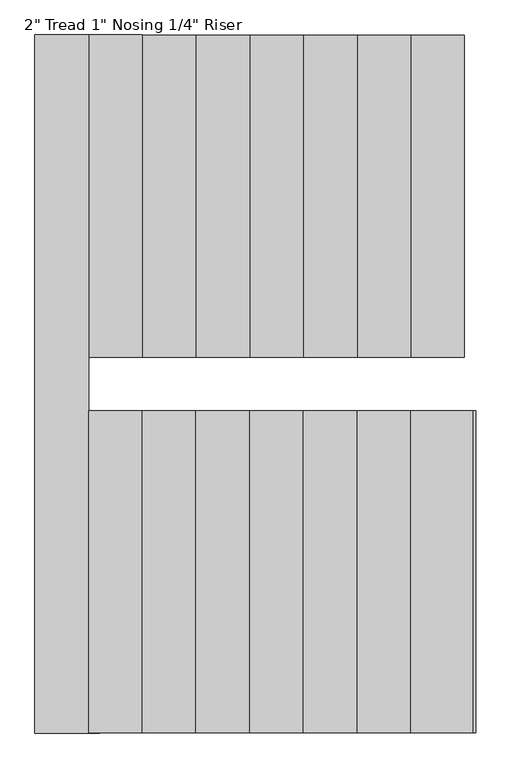
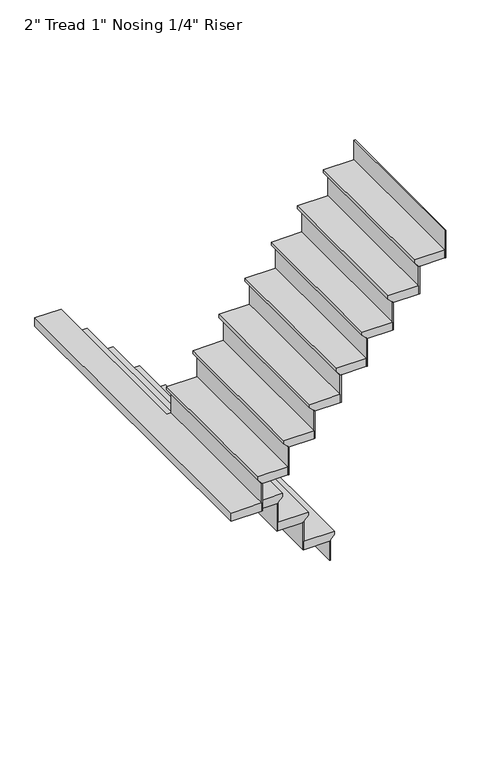
"""IFC4 building model written with IfcOpenShell, lengths in millimetres: stair flight geometry."""

from ifc_helpers import new_model, si_unit, origin, place, context, project, spatial, faceted_brep, source, transform, mapped, element, save


def stair_flight_173d3475(model_context):
    return source(origin(), model_context, "Body", "Brep", [
        faceted_brep([(3632.2, 10909.3, 6246.2833333), (3632.2, 10909.3, 6265.3333333), (3632.2, 9994.9, 6265.3333333), (3632.2, 9994.9, 6246.2833333), (3606.8, 10909.3, 6220.8833333), (3606.8, 9994.9, 6220.8833333), (3454.4, 10909.3, 6265.3333333), (3454.4, 9994.9, 6265.3333333), (3606.8, 9994.9, 6214.5333333), (3454.4, 9994.9, 6214.5333333), (3454.4, 10909.3, 6214.5333333), (3606.8, 10909.3, 6214.5333333)], [[[0, 1, 2, 3]], [[4, 0, 3, 5]], [[2, 1, 6, 7]], [[8, 9, 10, 11]], [[2, 7, 9, 8, 5, 3]], [[8, 11, 4, 5]], [[6, 1, 0, 4, 11, 10]], [[7, 6, 10, 9]]]),
        faceted_brep([(3606.8, 10909.3, 6214.5333333), (3606.8, 10909.3, 6096.0), (3600.45, 10909.3, 6096.0), (3600.45, 10909.3, 6214.5333333), (3606.8, 9994.9, 6214.5333333), (3600.45, 9994.9, 6214.5333333), (3600.45, 9994.9, 6096.0), (3606.8, 9994.9, 6096.0)], [[[0, 1, 2, 3]], [[4, 5, 6, 7]], [[1, 0, 4, 7]], [[2, 1, 7, 6]], [[3, 2, 6, 5]], [[0, 3, 5, 4]]]),
        faceted_brep([(3454.4, 10909.3, 6383.8666667), (3454.4, 10909.3, 6214.5333333), (3448.05, 10909.3, 6214.5333333), (3448.05, 10909.3, 6383.8666667), (3454.4, 9994.9, 6383.8666667), (3448.05, 9994.9, 6383.8666667), (3448.05, 9994.9, 6214.5333333), (3454.4, 9994.9, 6214.5333333)], [[[0, 1, 2, 3]], [[4, 5, 6, 7]], [[1, 0, 4, 7]], [[2, 1, 7, 6]], [[3, 2, 6, 5]], [[0, 3, 5, 4]]]),
        faceted_brep([(3479.8, 9994.9, 6434.6666667), (3479.8, 10909.3, 6434.6666667), (3302.0, 10909.3, 6434.6666667), (3302.0, 9994.9, 6434.6666667), (3454.4, 9994.9, 6383.8666667), (3302.0, 9994.9, 6383.8666667), (3302.0, 10909.3, 6383.8666667), (3454.4, 10909.3, 6383.8666667), (3454.4, 9994.9, 6390.2166667), (3479.8, 9994.9, 6415.6166667), (3454.4, 10909.3, 6390.2166667), (3479.8, 10909.3, 6415.6166667)], [[[0, 1, 2, 3]], [[4, 5, 6, 7]], [[0, 3, 5, 4, 8, 9]], [[4, 7, 10, 8]], [[2, 1, 11, 10, 7, 6]], [[3, 2, 6, 5]], [[11, 1, 0, 9]], [[10, 11, 9, 8]]]),
        faceted_brep([(3302.0, 10909.3, 6553.2), (3302.0, 10909.3, 6383.8666667), (3295.65, 10909.3, 6383.8666667), (3295.65, 10909.3, 6553.2), (3302.0, 9994.9, 6553.2), (3295.65, 9994.9, 6553.2), (3295.65, 9994.9, 6383.8666667), (3302.0, 9994.9, 6383.8666667)], [[[0, 1, 2, 3]], [[4, 5, 6, 7]], [[1, 0, 4, 7]], [[2, 1, 7, 6]], [[3, 2, 6, 5]], [[0, 3, 5, 4]]]),
        faceted_brep([(3327.4, 9994.9, 6604.0), (3327.4, 10909.3, 6604.0), (3149.6, 10909.3, 6604.0), (3149.6, 9994.9, 6604.0), (3302.0, 9994.9, 6553.2), (3149.6, 9994.9, 6553.2), (3149.6, 10909.3, 6553.2), (3302.0, 10909.3, 6553.2), (3302.0, 9994.9, 6559.55), (3327.4, 9994.9, 6584.95), (3302.0, 10909.3, 6559.55), (3327.4, 10909.3, 6584.95)], [[[0, 1, 2, 3]], [[4, 5, 6, 7]], [[0, 3, 5, 4, 8, 9]], [[4, 7, 10, 8]], [[2, 1, 11, 10, 7, 6]], [[3, 2, 6, 5]], [[11, 1, 0, 9]], [[10, 11, 9, 8]]]),
        faceted_brep([(3149.6, 10909.3, 6722.5333333), (3149.6, 10909.3, 6553.2), (3143.25, 10909.3, 6553.2), (3143.25, 10909.3, 6722.5333333), (3149.6, 9994.9, 6722.5333333), (3143.25, 9994.9, 6722.5333333), (3143.25, 9994.9, 6553.2), (3149.6, 9994.9, 6553.2)], [[[0, 1, 2, 3]], [[4, 5, 6, 7]], [[1, 0, 4, 7]], [[2, 1, 7, 6]], [[3, 2, 6, 5]], [[0, 3, 5, 4]]]),
        faceted_brep([(3175.0, 9994.9, 6773.3333333), (3175.0, 10909.3, 6773.3333333), (2997.2, 10909.3, 6773.3333333), (2997.2, 9994.9, 6773.3333333), (3149.6, 9994.9, 6722.5333333), (2997.2, 9994.9, 6722.5333333), (2997.2, 10909.3, 6722.5333333), (3149.6, 10909.3, 6722.5333333), (3149.6, 9994.9, 6728.8833333), (3175.0, 9994.9, 6754.2833333), (3149.6, 10909.3, 6728.8833333), (3175.0, 10909.3, 6754.2833333)], [[[0, 1, 2, 3]], [[4, 5, 6, 7]], [[0, 3, 5, 4, 8, 9]], [[4, 7, 10, 8]], [[2, 1, 11, 10, 7, 6]], [[3, 2, 6, 5]], [[11, 1, 0, 9]], [[10, 11, 9, 8]]]),
        faceted_brep([(2997.2, 10909.3, 6891.8666667), (2997.2, 10909.3, 6722.5333333), (2990.85, 10909.3, 6722.5333333), (2990.85, 10909.3, 6891.8666667), (2997.2, 9994.9, 6891.8666667), (2990.85, 9994.9, 6891.8666667), (2990.85, 9994.9, 6722.5333333), (2997.2, 9994.9, 6722.5333333)], [[[0, 1, 2, 3]], [[4, 5, 6, 7]], [[1, 0, 4, 7]], [[2, 1, 7, 6]], [[3, 2, 6, 5]], [[0, 3, 5, 4]]]),
        faceted_brep([(3022.6, 9994.9, 6942.6666667), (3022.6, 10909.3, 6942.6666667), (2844.8, 10909.3, 6942.6666667), (2844.8, 9994.9, 6942.6666667), (2997.2, 9994.9, 6891.8666667), (2844.8, 9994.9, 6891.8666667), (2844.8, 10909.3, 6891.8666667), (2997.2, 10909.3, 6891.8666667), (2997.2, 9994.9, 6898.2166667), (3022.6, 9994.9, 6923.6166667), (2997.2, 10909.3, 6898.2166667), (3022.6, 10909.3, 6923.6166667)], [[[0, 1, 2, 3]], [[4, 5, 6, 7]], [[0, 3, 5, 4, 8, 9]], [[4, 7, 10, 8]], [[2, 1, 11, 10, 7, 6]], [[3, 2, 6, 5]], [[11, 1, 0, 9]], [[10, 11, 9, 8]]]),
        faceted_brep([(2844.8, 10909.3, 7061.2), (2844.8, 10909.3, 6891.8666667), (2838.45, 10909.3, 6891.8666667), (2838.45, 10909.3, 7061.2), (2844.8, 9994.9, 7061.2), (2838.45, 9994.9, 7061.2), (2838.45, 9994.9, 6891.8666667), (2844.8, 9994.9, 6891.8666667)], [[[0, 1, 2, 3]], [[4, 5, 6, 7]], [[1, 0, 4, 7]], [[2, 1, 7, 6]], [[3, 2, 6, 5]], [[0, 3, 5, 4]]]),
        faceted_brep([(2870.2, 9994.9, 7112.0), (2870.2, 10909.3, 7112.0), (2692.4, 10909.3, 7112.0), (2692.4, 9994.9, 7112.0), (2844.8, 9994.9, 7061.2), (2692.4, 9994.9, 7061.2), (2692.4, 10909.3, 7061.2), (2844.8, 10909.3, 7061.2), (2844.8, 9994.9, 7067.55), (2870.2, 9994.9, 7092.95), (2844.8, 10909.3, 7067.55), (2870.2, 10909.3, 7092.95)], [[[0, 1, 2, 3]], [[4, 5, 6, 7]], [[0, 3, 5, 4, 8, 9]], [[4, 7, 10, 8]], [[2, 1, 11, 10, 7, 6]], [[3, 2, 6, 5]], [[11, 1, 0, 9]], [[10, 11, 9, 8]]]),
        faceted_brep([(2692.4, 10909.3, 7230.5333333), (2692.4, 10909.3, 7061.2), (2686.05, 10909.3, 7061.2), (2686.05, 10909.3, 7230.5333333), (2692.4, 9994.9, 7230.5333333), (2686.05, 9994.9, 7230.5333333), (2686.05, 9994.9, 7061.2), (2692.4, 9994.9, 7061.2)], [[[0, 1, 2, 3]], [[4, 5, 6, 7]], [[1, 0, 4, 7]], [[2, 1, 7, 6]], [[3, 2, 6, 5]], [[0, 3, 5, 4]]]),
        faceted_brep([(2717.8, 9994.9, 7281.3333333), (2717.8, 10909.3, 7281.3333333), (2540.0, 10909.3, 7281.3333333), (2540.0, 9994.9, 7281.3333333), (2692.4, 9994.9, 7230.5333333), (2540.0, 9994.9, 7230.5333333), (2540.0, 10909.3, 7230.5333333), (2692.4, 10909.3, 7230.5333333), (2692.4, 9994.9, 7236.8833333), (2717.8, 9994.9, 7262.2833333), (2692.4, 10909.3, 7236.8833333), (2717.8, 10909.3, 7262.2833333)], [[[0, 1, 2, 3]], [[4, 5, 6, 7]], [[0, 3, 5, 4, 8, 9]], [[4, 7, 10, 8]], [[2, 1, 11, 10, 7, 6]], [[3, 2, 6, 5]], [[11, 1, 0, 9]], [[10, 11, 9, 8]]]),
        faceted_brep([(2540.0, 10909.3, 7399.8666667), (2540.0, 10909.3, 7230.5333333), (2533.65, 10909.3, 7230.5333333), (2533.65, 10909.3, 7399.8666667), (2540.0, 9994.9, 7399.8666667), (2533.65, 9994.9, 7399.8666667), (2533.65, 9994.9, 7230.5333333), (2540.0, 9994.9, 7230.5333333)], [[[0, 1, 2, 3]], [[4, 5, 6, 7]], [[1, 0, 4, 7]], [[2, 1, 7, 6]], [[3, 2, 6, 5]], [[0, 3, 5, 4]]]),
        faceted_brep([(2590.8, 9842.5, 7450.6666667), (2565.4, 9842.5, 7450.6666667), (2565.4, 10909.3, 7450.6666667), (2413.0, 10909.3, 7450.6666667), (2413.0, 8928.1, 7450.6666667), (2590.8, 8928.1, 7450.6666667), (2565.4, 9842.5, 7399.8666667), (2590.8, 9842.5, 7399.8666667), (2590.8, 8928.1, 7399.8666667), (2413.0, 8928.1, 7399.8666667), (2413.0, 10909.3, 7399.8666667), (2540.0, 10909.3, 7399.8666667), (2540.0, 9994.9, 7399.8666667), (2565.4, 9994.9, 7399.8666667), (2565.4, 9994.9, 7431.6166667), (2565.4, 10909.3, 7431.6166667), (2540.0, 9994.9, 7406.2166667), (2540.0, 10909.3, 7406.2166667)], [[[0, 1, 2, 3, 4, 5]], [[6, 7, 8, 9, 10, 11, 12, 13]], [[1, 0, 7, 6]], [[2, 1, 6, 13, 14, 15]], [[13, 12, 16, 14]], [[12, 11, 17, 16]], [[3, 2, 15, 17, 11, 10]], [[4, 3, 10, 9]], [[5, 4, 9, 8]], [[0, 5, 8, 7]], [[17, 15, 14, 16]]]),
        faceted_brep([(2590.8, 8928.1, 7569.2), (2590.8, 8928.1, 7399.8666667), (2597.15, 8928.1, 7399.8666667), (2597.15, 8928.1, 7569.2), (2590.8, 9842.5, 7569.2), (2597.15, 9842.5, 7569.2), (2597.15, 9842.5, 7399.8666667), (2590.8, 9842.5, 7399.8666667)], [[[0, 1, 2, 3]], [[4, 5, 6, 7]], [[1, 0, 4, 7]], [[2, 1, 7, 6]], [[3, 2, 6, 5]], [[0, 3, 5, 4]]]),
        faceted_brep([(2565.4, 9842.5, 7620.0), (2565.4, 8928.1, 7620.0), (2743.2, 8928.1, 7620.0), (2743.2, 9842.5, 7620.0), (2590.8, 9842.5, 7569.2), (2743.2, 9842.5, 7569.2), (2743.2, 8928.1, 7569.2), (2590.8, 8928.1, 7569.2), (2590.8, 9842.5, 7575.55), (2565.4, 9842.5, 7600.95), (2590.8, 8928.1, 7575.55), (2565.4, 8928.1, 7600.95)], [[[0, 1, 2, 3]], [[4, 5, 6, 7]], [[0, 3, 5, 4, 8, 9]], [[4, 7, 10, 8]], [[2, 1, 11, 10, 7, 6]], [[3, 2, 6, 5]], [[11, 1, 0, 9]], [[10, 11, 9, 8]]]),
        faceted_brep([(2743.2, 8928.1, 7738.5333333), (2743.2, 8928.1, 7569.2), (2749.55, 8928.1, 7569.2), (2749.55, 8928.1, 7738.5333333), (2743.2, 9842.5, 7738.5333333), (2749.55, 9842.5, 7738.5333333), (2749.55, 9842.5, 7569.2), (2743.2, 9842.5, 7569.2)], [[[0, 1, 2, 3]], [[4, 5, 6, 7]], [[1, 0, 4, 7]], [[2, 1, 7, 6]], [[3, 2, 6, 5]], [[0, 3, 5, 4]]]),
        faceted_brep([(2717.8, 9842.5, 7789.3333333), (2717.8, 8928.1, 7789.3333333), (2895.6, 8928.1, 7789.3333333), (2895.6, 9842.5, 7789.3333333), (2743.2, 9842.5, 7738.5333333), (2895.6, 9842.5, 7738.5333333), (2895.6, 8928.1, 7738.5333333), (2743.2, 8928.1, 7738.5333333), (2743.2, 9842.5, 7744.8833333), (2717.8, 9842.5, 7770.2833333), (2743.2, 8928.1, 7744.8833333), (2717.8, 8928.1, 7770.2833333)], [[[0, 1, 2, 3]], [[4, 5, 6, 7]], [[0, 3, 5, 4, 8, 9]], [[4, 7, 10, 8]], [[2, 1, 11, 10, 7, 6]], [[3, 2, 6, 5]], [[11, 1, 0, 9]], [[10, 11, 9, 8]]]),
        faceted_brep([(2895.6, 8928.1, 7907.8666667), (2895.6, 8928.1, 7738.5333333), (2901.95, 8928.1, 7738.5333333), (2901.95, 8928.1, 7907.8666667), (2895.6, 9842.5, 7907.8666667), (2901.95, 9842.5, 7907.8666667), (2901.95, 9842.5, 7738.5333333), (2895.6, 9842.5, 7738.5333333)], [[[0, 1, 2, 3]], [[4, 5, 6, 7]], [[1, 0, 4, 7]], [[2, 1, 7, 6]], [[3, 2, 6, 5]], [[0, 3, 5, 4]]]),
        faceted_brep([(2870.2, 9842.5, 7958.6666667), (2870.2, 8928.1, 7958.6666667), (3048.0, 8928.1, 7958.6666667), (3048.0, 9842.5, 7958.6666667), (2895.6, 9842.5, 7907.8666667), (3048.0, 9842.5, 7907.8666667), (3048.0, 8928.1, 7907.8666667), (2895.6, 8928.1, 7907.8666667), (2895.6, 9842.5, 7914.2166667), (2870.2, 9842.5, 7939.6166667), (2895.6, 8928.1, 7914.2166667), (2870.2, 8928.1, 7939.6166667)], [[[0, 1, 2, 3]], [[4, 5, 6, 7]], [[0, 3, 5, 4, 8, 9]], [[4, 7, 10, 8]], [[2, 1, 11, 10, 7, 6]], [[3, 2, 6, 5]], [[11, 1, 0, 9]], [[10, 11, 9, 8]]]),
        faceted_brep([(3048.0, 8928.1, 8077.2), (3048.0, 8928.1, 7907.8666667), (3054.35, 8928.1, 7907.8666667), (3054.35, 8928.1, 8077.2), (3048.0, 9842.5, 8077.2), (3054.35, 9842.5, 8077.2), (3054.35, 9842.5, 7907.8666667), (3048.0, 9842.5, 7907.8666667)], [[[0, 1, 2, 3]], [[4, 5, 6, 7]], [[1, 0, 4, 7]], [[2, 1, 7, 6]], [[3, 2, 6, 5]], [[0, 3, 5, 4]]]),
        faceted_brep([(3022.6, 9842.5, 8128.0), (3022.6, 8928.1, 8128.0), (3200.4, 8928.1, 8128.0), (3200.4, 9842.5, 8128.0), (3048.0, 9842.5, 8077.2), (3200.4, 9842.5, 8077.2), (3200.4, 8928.1, 8077.2), (3048.0, 8928.1, 8077.2), (3048.0, 9842.5, 8083.55), (3022.6, 9842.5, 8108.95), (3048.0, 8928.1, 8083.55), (3022.6, 8928.1, 8108.95)], [[[0, 1, 2, 3]], [[4, 5, 6, 7]], [[0, 3, 5, 4, 8, 9]], [[4, 7, 10, 8]], [[2, 1, 11, 10, 7, 6]], [[3, 2, 6, 5]], [[11, 1, 0, 9]], [[10, 11, 9, 8]]]),
        faceted_brep([(3200.4, 8928.1, 8246.5333333), (3200.4, 8928.1, 8077.2), (3206.75, 8928.1, 8077.2), (3206.75, 8928.1, 8246.5333333), (3200.4, 9842.5, 8246.5333333), (3206.75, 9842.5, 8246.5333333), (3206.75, 9842.5, 8077.2), (3200.4, 9842.5, 8077.2)], [[[0, 1, 2, 3]], [[4, 5, 6, 7]], [[1, 0, 4, 7]], [[2, 1, 7, 6]], [[3, 2, 6, 5]], [[0, 3, 5, 4]]]),
        faceted_brep([(3175.0, 9842.5, 8297.3333333), (3175.0, 8928.1, 8297.3333333), (3352.8, 8928.1, 8297.3333333), (3352.8, 9842.5, 8297.3333333), (3200.4, 9842.5, 8246.5333333), (3352.8, 9842.5, 8246.5333333), (3352.8, 8928.1, 8246.5333333), (3200.4, 8928.1, 8246.5333333), (3200.4, 9842.5, 8252.8833333), (3175.0, 9842.5, 8278.2833333), (3200.4, 8928.1, 8252.8833333), (3175.0, 8928.1, 8278.2833333)], [[[0, 1, 2, 3]], [[4, 5, 6, 7]], [[0, 3, 5, 4, 8, 9]], [[4, 7, 10, 8]], [[2, 1, 11, 10, 7, 6]], [[3, 2, 6, 5]], [[11, 1, 0, 9]], [[10, 11, 9, 8]]]),
        faceted_brep([(3352.8, 8928.1, 8415.8666667), (3352.8, 8928.1, 8246.5333333), (3359.15, 8928.1, 8246.5333333), (3359.15, 8928.1, 8415.8666667), (3352.8, 9842.5, 8415.8666667), (3359.15, 9842.5, 8415.8666667), (3359.15, 9842.5, 8246.5333333), (3352.8, 9842.5, 8246.5333333)], [[[0, 1, 2, 3]], [[4, 5, 6, 7]], [[1, 0, 4, 7]], [[2, 1, 7, 6]], [[3, 2, 6, 5]], [[0, 3, 5, 4]]]),
        faceted_brep([(3327.4, 9842.5, 8466.6666667), (3327.4, 8928.1, 8466.6666667), (3505.2, 8928.1, 8466.6666667), (3505.2, 9842.5, 8466.6666667), (3352.8, 9842.5, 8415.8666667), (3505.2, 9842.5, 8415.8666667), (3505.2, 8928.1, 8415.8666667), (3352.8, 8928.1, 8415.8666667), (3352.8, 9842.5, 8422.2166667), (3327.4, 9842.5, 8447.6166667), (3352.8, 8928.1, 8422.2166667), (3327.4, 8928.1, 8447.6166667)], [[[0, 1, 2, 3]], [[4, 5, 6, 7]], [[0, 3, 5, 4, 8, 9]], [[4, 7, 10, 8]], [[2, 1, 11, 10, 7, 6]], [[3, 2, 6, 5]], [[11, 1, 0, 9]], [[10, 11, 9, 8]]]),
        faceted_brep([(3505.2, 8928.1, 8585.2), (3505.2, 8928.1, 8415.8666667), (3511.55, 8928.1, 8415.8666667), (3511.55, 8928.1, 8585.2), (3505.2, 9842.5, 8585.2), (3511.55, 9842.5, 8585.2), (3511.55, 9842.5, 8415.8666667), (3505.2, 9842.5, 8415.8666667)], [[[0, 1, 2, 3]], [[4, 5, 6, 7]], [[1, 0, 4, 7]], [[2, 1, 7, 6]], [[3, 2, 6, 5]], [[0, 3, 5, 4]]]),
        faceted_brep([(3657.6, 8928.1, 8754.5333333), (3657.6, 8928.1, 8585.2), (3663.95, 8928.1, 8585.2), (3663.95, 8928.1, 8754.5333333), (3657.6, 9842.5, 8754.5333333), (3663.95, 9842.5, 8754.5333333), (3663.95, 9842.5, 8585.2), (3657.6, 9842.5, 8585.2)], [[[0, 1, 2, 3]], [[4, 5, 6, 7]], [[1, 0, 4, 7]], [[2, 1, 7, 6]], [[3, 2, 6, 5]], [[0, 3, 5, 4]]]),
        faceted_brep([(3479.8, 9842.5, 8636.0), (3479.8, 8928.1, 8636.0), (3657.6, 8928.1, 8636.0), (3657.6, 9842.5, 8636.0), (3505.2, 9842.5, 8585.2), (3657.6, 9842.5, 8585.2), (3657.6, 8928.1, 8585.2), (3505.2, 8928.1, 8585.2), (3505.2, 9842.5, 8591.55), (3479.8, 9842.5, 8616.95), (3505.2, 8928.1, 8591.55), (3479.8, 8928.1, 8616.95)], [[[0, 1, 2, 3]], [[4, 5, 6, 7]], [[0, 3, 5, 4, 8, 9]], [[4, 7, 10, 8]], [[2, 1, 11, 10, 7, 6]], [[3, 2, 6, 5]], [[11, 1, 0, 9]], [[10, 11, 9, 8]]]),
    ])


if __name__ == "__main__":
    model = new_model("IFC4")
    model_context = context("Model", 3, world=origin())
    ifc_project = project(units=[si_unit("LENGTHUNIT", "METRE", prefix="MILLI")], contexts=[model_context])
    site = spatial("IfcSite", under=ifc_project)
    building = spatial("IfcBuilding", under=site)
    placement = place(None, origin())
    stair_flight_shape = stair_flight_173d3475(model_context)
    element("IfcStairFlight", 1, ObjectType="2\" Tread 1\" Nosing 1/4\" Riser", at=placement, inside=building, context=model_context, shape_type="MappedRepresentation", body=[
        mapped(stair_flight_shape, transform((0.0, 0.0, 0.0), x_axis=(1.0, 0.0, 0.0), y_axis=(0.0, 1.0, 0.0), z_axis=(0.0, 0.0, 1.0))),
    ])
    save(model, "model.ifc")
